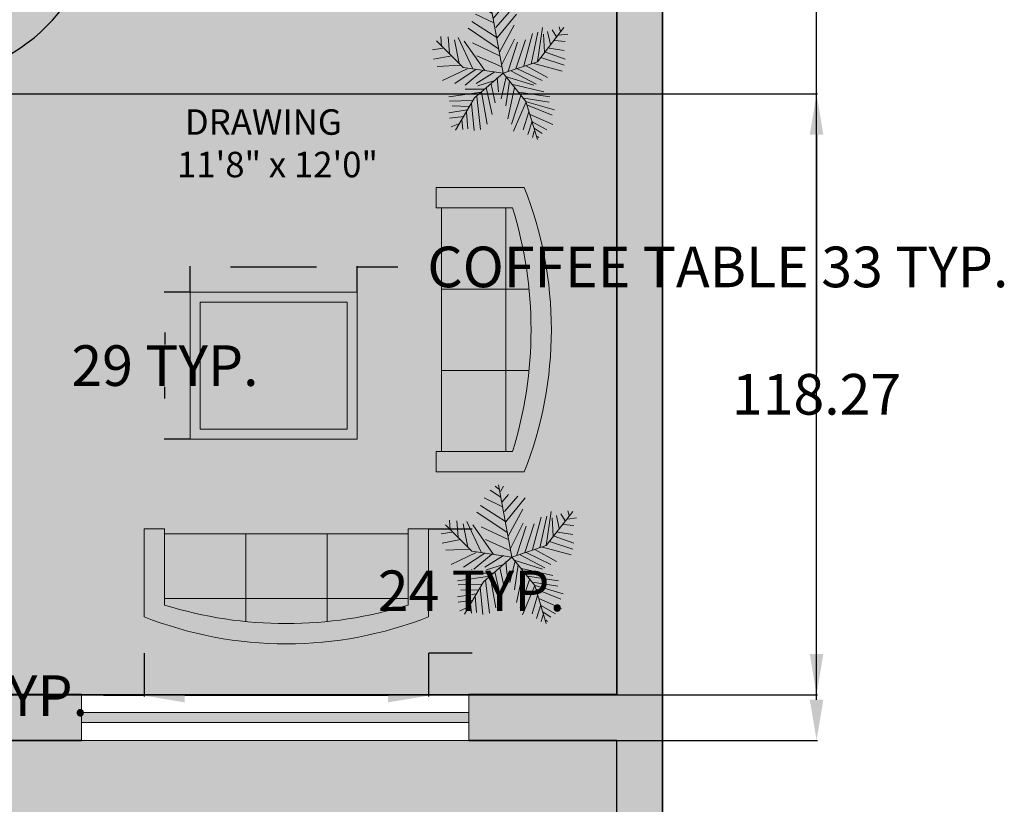
# Model space of a CAD drawing. Units: inches. Extents: x 389 to 971, y 148 to 870.
# Tile 6 of 14: x 722 to 916, y 273 to 428. Entities that reach past the tile are written whole.
import ezdxf

# ---------------------------------------------------------------- set-up
doc = ezdxf.new("R2010")
doc.units = ezdxf.units.IN
doc.header["$MEASUREMENT"] = 0
for name, color, linetype, lineweight in [('A-ANNO-DIMS', 2, 'Continuous', 18), ('A-AREA-IDEN', 7, 'Continuous', 18), ('A-DOOR', 4, 'Continuous', 25), ('A-FLOR-BASE-PATT', 8, 'Continuous', 13), ('A-FURN', 8, 'Continuous', 18), ('A-GLAZ', 4, 'Continuous', 18), ('A-WALL', 7, 'Continuous', 35), ('C-PROP', 7, 'Continuous', 35), ('L-GRND-BASE-PATT', 8, 'Continuous', 13), ('L-PLNT', 3, 'Continuous', 13), ('L-WALL', 7, 'Continuous', 30)]:
    doc.layers.add(name, color=color, linetype=linetype, lineweight=lineweight)
for name, color, linetype, lineweight, true_color in [('A-FURN-SURF-PATT', 9, 'Continuous', 13, 0xd6bdce), ('A-GLAZ-PATT', 251, 'Continuous', 13, 0x6d5f6c), ('A-WALL-PATT', 18, 'Continuous', 13, 0x000000), ('L-GRND-PATT', 39, 'Continuous', 13, 0x603913)]:
    doc.layers.add(name, color=color, linetype=linetype, lineweight=lineweight, true_color=true_color)
doc.styles.get("Standard").update_dxf_attribs({"font": 'arial.ttf'})
doc.dimstyles.get("Standard").update_dxf_attribs({"dimtxt": 8, "dimasz": 8, "dimexe": 0.18, "dimexo": 0.0625, "dimgap": 0.09, "dimtad": 0, "dimtih": 1, "dimtoh": 1, "dimdec": 0, "dimzin": 0, "dimdsep": 46, "dimlunit": 3, "dimtxsty": 'Standard', "dimcen": 0.09, "dimadec": 0, "dimazin": 0, "dimtfac": 1, "dimtdec": 0, "dimtofl": 0, "dimtmove": 0, "dimatfit": 3, "dimfxl": 1, "dimtolj": 1, "dimtzin": 0, "dimarcsym": 0})

# ---------------------------------------------------------------- blocks, each defined once
blk = doc.blocks.new('*U5')
for p, q in [((0, 0), (0, -6)), ((28, 0), (28, -6))]:
    blk.add_line(p, q)
blk.add_lwpolyline([(0, 0), (0, 28), (1.75, 28), (1.75, 0)], close=True)
blk.add_arc((0, 0), 28, 0, 90)
blk = doc.blocks.new('Sofa - Roundback 7 ft.')
for p, q in [((-12.00002, -32.4421), (-12.00003, -6.5971)), ((11.99997, -32.4421), (11.99998, -6.5971)), ((-36.000027, -34), (-36.000027, -11.4696)), ((35.99998, -34), (35.99998, -11.4696)), ((-35.999844, -13.3819), (35.9998, -13.3819)), ((-36.000027, -32.4421), (35.99998, -32.4421))]:
    blk.add_line(p, q)
for points in [[(-36.000027, -34), (-42.000027, -34), (-42.000027, -8)], [(41.99998, -8), (41.99998, -34), (35.99998, -34)]]:
    blk.add_lwpolyline(points)
for centre, radius, start, end in [((0, -114.25), 114.25, 68.43141, 111.5686), ((-0.00001, -127.1968), 121.1968, 72.72033, 107.2797)]:
    blk.add_arc(centre, radius, start, end)
blk = doc.blocks.new('*U19')
for p, q in [((-258.7244, 1362.456), (-332.3336, 1421.4348)), ((0, 0), (-266.7, 1447.8)), ((-231.1146, 1315.2628), (-166.7002, 1421.4348)), ((-185.1152, 1008.5578), (-553.1612, 1185.4942)), ((-221.9198, 1197.3052), (-433.5526, 1338.8594)), ((-194.31, 1102.9442), (-65.4812, 1256.284)), ((-148.3106, 914.1968), (118.5418, 1220.9018)), ((-129.8956, 701.8528), (265.7602, 1185.4942)), ((-129.8956, 713.6638), (-626.7704, 1032.1544)), ((-93.091, 489.5342), (-700.3796, 902.3858)), ((-74.7014, 418.7444), (219.7608, 961.39)), ((412.9786, 147.447), (587.8068, 796.2392)), ((560.197, 182.8292), (698.2206, 819.8358)), ((685.8, 228.6), (1219.2, 914.4)), ((689.0258, 230.0224), (790.2448, 914.1968)), ((891.4384, 831.6214), (946.658, 572.1096)), ((983.4626, 867.0036), (1066.2666, 725.4494)), ((1121.4862, 925.9824), (1149.0706, 831.6214)), ((-800.1, 114.3), (-1333.5, 647.7)), ((-1234.059, 536.7274), (-1252.4486, 737.2604)), ((-1105.2302, 725.4494), (-1077.6458, 395.1732)), ((-976.4268, 666.4706), (-884.4026, 194.6402)), ((-902.8176, 713.6638), (-617.5756, 100.2538)), ((-369.1382, 53.086), (-783.1836, 642.874)), ((-617.5756, 607.4918), (-74.7014, 347.98)), ((-28.6766, 171.0436), (228.9556, 678.2816)), ((100.1268, 41.275), (284.1498, 619.2774)), ((256.5654, 88.4682), (449.7832, 666.4706)), ((808.6344, 784.4282), (827.0494, 418.7444)), ((1029.462, 654.685), (1241.0948, 631.0884)), ((1112.2914, 760.8316), (1296.3144, 784.4282)), ((-1206.4492, 501.3198), (-1418.082, 465.9376)), ((845.439, 418.7444), (1241.0948, 277.1902)), ((919.0482, 501.3198), (1222.6798, 454.152)), ((-1031.621, 347.98), (-1399.667, 277.1902)), ((-525.5514, 347.98), (-28.6766, 123.8504)), ((0, 0), (685.8, 228.6)), ((753.4148, 312.5978), (1222.6798, 159.2326)), ((-847.598, 159.2326), (-1326.0578, 135.636)), ((-718.7946, 88.4682), (-1215.644, -147.447)), ((-543.9664, 76.6572), (-967.2066, -206.4512)), ((0, 0), (-800.1, 114.3)), ((-405.9428, 53.086), (-764.794, -241.8334)), ((0, 0), (-571.5, -495.3)), ((-166.7002, 29.4894), (-543.9664, -206.4512)), ((0, 0), (457.2, -571.5)), ((164.5412, 41.275), (661.416, -218.2368)), ((284.1498, 88.4682), (781.0246, -147.447)), ((458.978, 147.447), (891.4384, -88.4682)), ((615.4166, 194.6402), (1185.8752, 41.275)), ((-166.7002, -147.447), (-507.1618, -253.619)), ((-120.7008, -88.4682), (-93.091, -371.5766)), ((63.3222, -76.6826), (-37.8714, -513.1308)), ((44.9326, -64.897), (615.4166, -241.8334)), ((127.7366, -159.258), (54.1274, -654.685)), ((-442.7474, -383.3876), (-1086.8406, -477.7486)), ((-387.5278, -324.4088), (-764.794, -324.4088)), ((-433.5526, -383.3876), (-323.1134, -1020.3688)), ((-341.5284, -289.0012), (-221.9198, -831.6214)), ((-240.3094, -218.2368), (-157.5054, -595.7062)), ((228.9556, -289.0012), (90.932, -914.1968)), ((192.151, -230.0224), (817.8292, -371.5766)), ((311.7596, -383.3876), (937.4378, -477.7486)), ((-617.5756, -548.5384), (-1077.6458, -560.324)), ((-571.5, -495.3), (-952.5, -1143)), ((-525.5514, -465.963), (-451.9422, -1126.5408)), ((357.759, -430.5554), (164.5412, -1020.3688)), ((458.978, -572.1096), (210.5406, -1161.923)), ((412.9786, -501.3452), (919.0482, -583.9206)), ((457.2, -571.5), (685.8, -1333.5)), ((468.1982, -572.1096), (1029.462, -737.2604)), ((-718.7946, -737.2604), (-1086.8406, -796.2392)), ((-681.9646, -666.496), (-1022.4262, -654.685)), ((-737.1842, -784.4536), (-709.5744, -1114.7298)), ((-635.9652, -607.5172), (-580.771, -1150.1374)), ((514.1976, -772.6426), (403.7838, -1138.3264)), ((486.5878, -642.8994), (983.4626, -843.4324)), ((-783.1836, -867.029), (-1077.6458, -902.4112)), ((-829.2084, -937.7934), (-810.7934, -1126.5408)), ((578.612, -961.39), (495.7826, -1232.7128)), ((541.8074, -831.6214), (992.6574, -1032.1544)), ((578.612, -973.1756), (873.0488, -1138.3264)), ((-875.2078, -1008.5832), (-1040.8412, -1079.3476)), ((624.6114, -1161.923), (587.8068, -1291.6916)), ((624.6114, -1102.9442), (781.0246, -1209.1162)), ((679.8056, -1268.095), (716.6102, -1291.6916))]:
    blk.add_line(p, q)
blk = doc.blocks.new('COFFEE-TABLE-RECT')
for points in [[(0, 28.98), (32.94, 28.98), (32.94, 0), (0, 0)], [(2, 26.98), (30.94, 26.98), (30.94, 2), (2, 2)]]:
    blk.add_lwpolyline(points, close=True)
blk = doc.blocks.new('*D38')
at = {"layer": 'A-ANNO-DIMS', "color": 0, "lineweight": -2, "transparency": 16777216}
for p, q in [((746.14, 302.8), (746.14, 294.28)), ((802.17, 302.8), (802.17, 294.28)), ((746.14, 294.46), (738.14, 294.46)), ((794.17, 294.46), (754.14, 294.46))]:
    blk.add_line(p, q, dxfattribs=at)
at = {"layer": 'A-ANNO-DIMS', "color": 0, "transparency": 16777216}
for points in [[(754.14, 295.79), (754.14, 293.12), (746.14, 294.46)], [(794.17, 295.79), (794.17, 293.12), (802.17, 294.46)]]:
    blk.add_solid(points, dxfattribs=at)
at = {"layer": 'Defpoints', "color": 0, "transparency": 16777216}
for p in [(746.14, 302.86), (802.17, 302.86), (746.14, 294.46)]:
    blk.add_point(p, dxfattribs=at)
at = {"layer": 'A-ANNO-DIMS', "color": 0, "transparency": 16777216, "insert": (701.83, 294.46), "char_height": 8, "attachment_point": 5}
blk.add_mtext('\\A1;SOFA 56 TYP.', dxfattribs=at)
blk = doc.blocks.new('*D39')
at = {"layer": 'A-ANNO-DIMS', "color": 0, "lineweight": -2, "transparency": 16777216}
for p, q in [((802.23, 327.32), (810.76, 327.32)), ((810.58, 319.32), (810.58, 319.2)), ((810.58, 310.86), (810.58, 310.98)), ((802.23, 302.86), (810.76, 302.86))]:
    blk.add_line(p, q, dxfattribs=at)
at = {"layer": 'A-ANNO-DIMS', "color": 0, "transparency": 16777216}
for points in [[(809.24, 319.32), (811.91, 319.32), (810.58, 327.32)], [(809.24, 310.86), (811.91, 310.86), (810.58, 302.86)]]:
    blk.add_solid(points, dxfattribs=at)
at = {"layer": 'Defpoints', "color": 0, "transparency": 16777216}
for p in [(802.17, 327.32), (802.17, 302.86), (810.58, 302.86)]:
    blk.add_point(p, dxfattribs=at)
at = {"layer": 'A-ANNO-DIMS', "color": 0, "transparency": 16777216, "insert": (810.58, 315.09), "char_height": 8, "attachment_point": 5}
blk.add_mtext('\\A1;24 TYP.', dxfattribs=at)
blk = doc.blocks.new('*D42')
at = {"layer": 'A-ANNO-DIMS', "color": 0, "lineweight": -2, "transparency": 16777216}
for p, q in [((755.19, 373.98), (755.19, 379.04)), ((763.19, 378.86), (780.12, 378.86)), ((788.12, 373.98), (788.12, 379.04)), ((788.12, 378.86), (796.12, 378.86))]:
    blk.add_line(p, q, dxfattribs=at)
at = {"layer": 'A-ANNO-DIMS', "color": 0, "transparency": 16777216}
for points in [[(763.19, 380.19), (763.19, 377.52), (755.19, 378.86)], [(780.12, 380.19), (780.12, 377.52), (788.12, 378.86)]]:
    blk.add_solid(points, dxfattribs=at)
at = {"layer": 'Defpoints', "color": 0, "transparency": 16777216}
for p in [(788.12, 378.86), (755.19, 373.92), (788.12, 373.92)]:
    blk.add_point(p, dxfattribs=at)
at = {"layer": 'A-ANNO-DIMS', "color": 0, "transparency": 16777216, "insert": (859.11, 378.86), "char_height": 8, "attachment_point": 5}
blk.add_mtext('\\A1;COFFEE TABLE 33 TYP.', dxfattribs=at)
blk = doc.blocks.new('*D43')
at = {"layer": 'A-ANNO-DIMS', "color": 0, "lineweight": -2, "transparency": 16777216}
for p, q in [((755.12, 373.92), (750.07, 373.92)), ((750.25, 365.92), (750.25, 363.6)), ((750.25, 352.94), (750.25, 355.25)), ((755.12, 344.94), (750.07, 344.94))]:
    blk.add_line(p, q, dxfattribs=at)
at = {"layer": 'A-ANNO-DIMS', "color": 0, "transparency": 16777216}
for points in [[(748.91, 365.92), (751.58, 365.92), (750.25, 373.92)], [(748.91, 352.94), (751.58, 352.94), (750.25, 344.94)]]:
    blk.add_solid(points, dxfattribs=at)
at = {"layer": 'Defpoints', "color": 0, "transparency": 16777216}
for p in [(750.25, 373.92), (755.19, 373.92), (755.19, 344.94)]:
    blk.add_point(p, dxfattribs=at)
at = {"layer": 'A-ANNO-DIMS', "color": 0, "transparency": 16777216, "insert": (750.25, 359.43), "char_height": 8, "attachment_point": 5}
blk.add_mtext('\\A1;29 TYP.', dxfattribs=at)
blk = doc.blocks.new('*D47')
at = {"layer": 'A-ANNO-DIMS', "color": 0, "lineweight": -2, "transparency": 16777216}
for p, q in [((848.28, 834.64), (878.72, 834.64)), ((878.54, 826.64), (878.54, 564.32)), ((878.54, 293.64), (878.54, 555.97)), ((839.28, 285.64), (878.72, 285.64))]:
    blk.add_line(p, q, dxfattribs=at)
at = {"layer": 'A-ANNO-DIMS', "color": 0, "transparency": 16777216}
for points in [[(877.21, 826.64), (879.87, 826.64), (878.54, 834.64)], [(877.21, 293.64), (879.87, 293.64), (878.54, 285.64)]]:
    blk.add_solid(points, dxfattribs=at)
at = {"layer": 'Defpoints', "color": 0, "transparency": 16777216}
for p in [(848.22, 834.64), (878.54, 834.64), (839.22, 285.64)]:
    blk.add_point(p, dxfattribs=at)
at = {"layer": 'A-ANNO-DIMS', "color": 0, "transparency": 16777216, "insert": (878.54, 560.14), "char_height": 8, "attachment_point": 5}
blk.add_mtext('\\A1;549', dxfattribs=at)
blk = doc.blocks.new('*D54')
at = {"layer": 'A-ANNO-DIMS', "color": 0, "lineweight": -2, "transparency": 16777216}
for p, q in [((690.28, 412.92), (878.72, 412.92)), ((878.54, 404.92), (878.54, 357.96)), ((878.54, 302.64), (878.54, 349.61)), ((690.28, 294.64), (878.72, 294.64))]:
    blk.add_line(p, q, dxfattribs=at)
at = {"layer": 'A-ANNO-DIMS', "color": 0, "transparency": 16777216}
for points in [[(877.21, 404.92), (879.87, 404.92), (878.54, 412.92)], [(877.21, 302.64), (879.87, 302.64), (878.54, 294.64)]]:
    blk.add_solid(points, dxfattribs=at)
at = {"layer": 'Defpoints', "color": 0, "transparency": 16777216}
for p in [(690.22, 412.92), (878.54, 412.92), (690.22, 294.64)]:
    blk.add_point(p, dxfattribs=at)
at = {"layer": 'A-ANNO-DIMS', "color": 0, "transparency": 16777216, "insert": (878.54, 353.78), "char_height": 8, "attachment_point": 5}
blk.add_mtext('\\A1;118.27', dxfattribs=at)

msp = doc.modelspace()

# ---------------------------------------------------------------- hatches: boundary and pattern name
at = {"layer": 'A-FLOR-BASE-PATT'}
h = msp.add_hatch(color=256, dxfattribs=at)
h.dxf.hatch_style = 1
h.paths.add_polyline_path([(634.6594, 428.4021), (634.6594, 427.0792), (634.6305, 427.0792, -0.40145271), (604.4225, 398.1652), (604.0817, 398.1199, -0.40145271), (632.0195, 371.3788), (632.0462, 371.3788), (632.0462, 370.1554), (604.387, 370.1554), (604.387, 366.7191), (640.0296, 366.7191), (640.0296, 321.4969, 1), (647.061, 321.4969), (647.061, 412.9189), (690.216, 412.9189), (690.216, 416.0006), (694.716, 416.0006), (702.2145, 416.0006, 0.39601219), (737.1392, 448.8066), (702.2145, 448.8066), (702.2145, 450.9936), (694.716, 450.9936), (690.216, 450.9936), (690.216, 466.6012), (708.7881, 466.6012), (708.7881, 462.1012), (784.6145, 462.1012), (784.6145, 466.6012), (794.216, 466.6012), (794.216, 591.6445), (708.5171, 591.6445), (708.5171, 596.1445), (708.5171, 602.9755, 0.39601219), (678.6314, 634.7912), (678.6314, 602.9755), (676.6391, 602.9755), (676.6391, 596.1445), (676.6391, 591.6445), (661.216, 591.6445), (661.216, 632.6445), (653.109, 632.6445), (653.109, 641.6445), (653.109, 642.1751), (651.6417, 642.1751), (651.6417, 675.6801, 0.40145271), (619.5719, 642.1751), (619.5719, 637.1445), (619.5147, 632.6445), (604.387, 632.6445), (604.387, 545.7317), (595.3894, 545.7317), (595.3894, 544.4199), (565.4338, 544.4199, 0.40145271), (595.3894, 515.7475), (599.887, 515.7475), (604.387, 515.7271), (604.387, 428.4021)])
h.paths.add_polyline_path([(721.8003, 493.9292), (725.0899, 493.9292), (725.0899, 493.075), (751.4065, 493.075), (751.4065, 493.9292), (754.6961, 493.9292), (754.6961, 479.6744, -0.26666697), (721.8003, 479.6744)], flags=16)
h.paths.add_polyline_path([(720.6421, 516.0583), (720.6421, 545.0393), (753.5806, 545.0393), (753.5806, 516.0583)], flags=16)
h.paths.add_polyline_path([(722.6421, 518.0583), (722.6421, 543.0393), (751.5806, 543.0393), (751.5806, 518.0583)], flags=0)
h.paths.add_polyline_path([(763.7396, 488.5801), (763.7822, 488.1156), (764.1436, 488.1761)], flags=16)
h.paths.add_polyline_path([(777.9011, 479.7417), (778.0475, 480.1886), (777.4745, 480.275)], flags=16)
h.paths.add_polyline_path([(762.3329, 503.5919), (762.3329, 507.1718), (763.2624, 507.1718), (763.2624, 550.1306), (762.3329, 550.1306), (762.3329, 553.7105), (777.8458, 553.7105, -0.19047621), (777.8458, 503.5919)], flags=16)
h.paths.add_polyline_path([(721.6097, 567.2898), (721.6097, 581.7362, -0.26666697), (754.9475, 581.7362), (754.9475, 567.2898), (751.6137, 567.2898), (751.6137, 568.1555), (724.9435, 568.1555), (724.9435, 567.2898)], flags=16)
h.paths.add_polyline_path([(774.6347, 521.4914), (774.6347, 535.811), (778.6837, 535.811, -0.04962821), (778.6837, 521.4914)], flags=0)
h.paths.add_polyline_path([(764.6624, 576.8996), (764.7454, 576.4742), (765.0717, 576.4903)], flags=16)
h.paths.add_polyline_path([(777.2772, 570.3652), (777.4444, 570.8756), (776.7899, 570.9743)], flags=16)
h.paths.add_polyline_path([(644.2892, 516.9956), (685.2491, 516.9956), (685.2491, 535.7223), (644.2892, 535.7223)], flags=24)
h = msp.add_hatch(color=256, dxfattribs=at)
h.dxf.hatch_style = 1
h.paths.add_polyline_path([(699.216, 294.6445), (733.8057, 294.6445), (810.0514, 294.6445), (839.216, 294.6445), (839.216, 457.6012), (784.6145, 457.6012), (784.6145, 462.1012), (708.7881, 462.1012), (708.7881, 457.6012), (699.216, 457.6012), (699.216, 450.9936), (702.2145, 450.9936), (737.2076, 450.9936), (737.2076, 448.8066), (737.1392, 448.8066, -0.39601219), (702.2145, 416.0006), (699.216, 416.0006)])
h.paths.add_polyline_path([(755.1859, 373.9163), (788.1244, 373.9163), (788.1244, 344.9352), (755.1859, 344.9352)], flags=16)
h.paths.add_polyline_path([(757.1859, 371.9163), (786.1244, 371.9163), (786.1244, 346.9352), (757.1859, 346.9352)], flags=0)
h.paths.add_polyline_path([(746.1376, 327.3223), (750.14, 327.3223), (750.14, 326.2831), (798.1694, 326.2831), (798.1694, 327.3223), (802.1718, 327.3223), (802.1718, 309.9784, -0.19047621), (746.1376, 309.9784)], flags=16)
h.paths.add_polyline_path([(782.1596, 313.5685), (782.1596, 309.0415, -0.04962821), (766.1498, 309.0415), (766.1498, 313.5685)], flags=0)
h.paths.add_polyline_path([(804.6838, 390.5197), (803.6446, 390.5197), (803.6446, 394.5221), (820.9885, 394.5221, -0.19047621), (820.9885, 338.4879), (803.6446, 338.4879), (803.6446, 342.4903), (804.6838, 342.4903)], flags=16)
h.paths.add_polyline_path([(817.3984, 358.5001), (817.3984, 374.5099), (821.9254, 374.5099, -0.04962821), (821.9254, 358.5001)], flags=0)
h.paths.add_polyline_path([(806.8707, 326.6963), (806.4254, 327.1416), (806.4724, 326.6297)], flags=16)
h.paths.add_polyline_path([(822.0328, 317.4008), (822.1942, 317.8933), (821.5626, 317.9885)], flags=16)
h.paths.add_polyline_path([(808.1446, 418.9737), (808.2247, 418.5632), (808.5395, 418.5787)], flags=16)
h.paths.add_polyline_path([(820.3159, 412.669), (820.4772, 413.1615), (819.8457, 413.2568)], flags=16)
h.paths.add_polyline_path([(750.6082, 393.6667), (791.5681, 393.6667), (791.5681, 412.3933), (750.6082, 412.3933)], flags=24)
at = {"layer": 'A-FURN-SURF-PATT'}
h = msp.add_hatch(color=256, dxfattribs=at)
h.dxf.hatch_style = 1
h.paths.add_polyline_path([(820.9885, 338.4879, 0.19047621), (820.9885, 394.5221), (803.6446, 394.5221), (803.6446, 390.5197), (818.6737, 390.5197, -0.15194781), (818.6737, 342.4903), (803.6446, 342.4903), (803.6446, 338.4879)])
h = msp.add_hatch(color=256, dxfattribs=at)
h.dxf.hatch_style = 1
h.paths.add_polyline_path([(817.3984, 374.5099), (817.3984, 390.5197), (804.6838, 390.5197), (804.6838, 374.5099)])
h = msp.add_hatch(color=256, dxfattribs=at)
h.dxf.hatch_style = 1
h.paths.add_polyline_path([(818.6737, 390.5197), (817.3984, 390.5197), (817.3984, 374.5099), (821.9254, 374.5099, 0.05064665)])
h = msp.add_hatch(color=256, dxfattribs=at)
h.dxf.hatch_style = 1
h.paths.add_polyline_path([(817.3984, 374.5099), (804.6838, 374.5099), (804.6838, 358.5001), (817.3984, 358.5001)])
h = msp.add_hatch(color=256, dxfattribs=at)
h.dxf.hatch_style = 1
h.paths.add_polyline_path([(821.9254, 374.5099), (817.3984, 374.5099), (817.3984, 358.5001), (821.9254, 358.5001, 0.04962821)])
h = msp.add_hatch(color=256, dxfattribs=at)
h.dxf.hatch_style = 1
h.paths.add_polyline_path([(788.1244, 373.9163), (755.1859, 373.9163), (755.1859, 344.9352), (788.1244, 344.9352)])
h.paths.add_polyline_path([(786.1244, 346.9352), (757.1859, 346.9352), (757.1859, 371.9163), (786.1244, 371.9163)], flags=16)
h = msp.add_hatch(color=256, dxfattribs=at)
h.dxf.hatch_style = 1
h.paths.add_polyline_path([(786.1244, 346.9352), (786.1244, 371.9163), (757.1859, 371.9163), (757.1859, 346.9352)])
h = msp.add_hatch(color=256, dxfattribs=at)
h.dxf.hatch_style = 1
h.paths.add_polyline_path([(804.6838, 342.4903), (817.3984, 342.4903), (817.3984, 358.5001), (804.6838, 358.5001)])
h = msp.add_hatch(color=256, dxfattribs=at)
h.dxf.hatch_style = 1
h.paths.add_polyline_path([(821.9254, 358.5001), (817.3984, 358.5001), (817.3984, 342.4903), (818.6737, 342.4903, 0.05064665)])
h = msp.add_hatch(color=256, dxfattribs=at)
h.dxf.hatch_style = 1
h.paths.add_polyline_path([(802.1718, 309.9784), (802.1718, 327.3223), (798.1694, 327.3223), (798.1694, 312.2932, -0.15194781), (750.14, 312.2932), (750.14, 327.3223), (746.1376, 327.3223), (746.1376, 309.9784, 0.19047621)])
h = msp.add_hatch(color=256, dxfattribs=at)
h.dxf.hatch_style = 1
h.paths.add_polyline_path([(750.14, 326.2831), (750.14, 313.5685), (766.1498, 313.5685), (766.1498, 326.2831)])
h = msp.add_hatch(color=256, dxfattribs=at)
h.dxf.hatch_style = 1
h.paths.add_polyline_path([(766.1498, 313.5685), (782.1596, 313.5685), (782.1596, 326.2831), (766.1498, 326.2831)])
h = msp.add_hatch(color=256, dxfattribs=at)
h.dxf.hatch_style = 1
h.paths.add_polyline_path([(798.1694, 313.5685), (798.1694, 326.2831), (782.1596, 326.2831), (782.1596, 313.5685)])
h = msp.add_hatch(color=256, dxfattribs=at)
h.dxf.hatch_style = 1
h.paths.add_polyline_path([(750.14, 313.5685), (750.14, 312.2932, 0.05064665), (766.1498, 309.0415), (766.1498, 313.5685)])
h = msp.add_hatch(color=256, dxfattribs=at)
h.dxf.hatch_style = 1
h.paths.add_polyline_path([(766.1498, 313.5685), (766.1498, 309.0415, 0.04962821), (782.1596, 309.0415), (782.1596, 313.5685)])
h = msp.add_hatch(color=256, dxfattribs=at)
h.dxf.hatch_style = 1
h.paths.add_polyline_path([(798.1694, 312.2932), (798.1694, 313.5685), (782.1596, 313.5685), (782.1596, 309.0415, 0.05064665)])
at = {"layer": 'A-GLAZ-PATT'}
h = msp.add_hatch(color=256, dxfattribs=at)
h.dxf.hatch_style = 1
h.paths.add_polyline_path([(733.8057, 291.1445), (733.8057, 289.1445), (810.0514, 289.1445), (810.0514, 291.1445)])
h = msp.add_hatch(color=256, dxfattribs=at)
h.dxf.hatch_style = 1
h.paths.add_polyline_path([(733.8057, 291.1445), (733.8057, 289.1445), (810.0514, 289.1445), (810.0514, 291.1445)])
h = msp.add_hatch(color=256, dxfattribs=at)
h.dxf.hatch_style = 1
h.paths.add_polyline_path([(810.0514, 289.1445), (810.0514, 291.1445), (733.8057, 291.1445), (733.8057, 289.1445)])
h = msp.add_hatch(color=256, dxfattribs=at)
h.dxf.hatch_style = 1
h.paths.add_polyline_path([(733.8057, 291.1445), (733.8057, 289.1445), (810.0514, 289.1445), (810.0514, 291.1445)])
h = msp.add_hatch(color=256, dxfattribs=at)
h.dxf.hatch_style = 1
h.paths.add_polyline_path([(733.8057, 291.1445), (733.8057, 289.1445), (810.0514, 289.1445), (810.0514, 291.1445)])
at = {"layer": 'A-WALL-PATT'}
h = msp.add_hatch(color=256, dxfattribs=at)
h.dxf.hatch_style = 1
h.paths.add_polyline_path([(432.216, 434.6445), (436.3673, 434.6445), (436.3673, 443.6445), (432.216, 443.6445), (432.216, 830.6445), (746.216, 830.6445), (746.216, 823.8175), (755.216, 823.8175), (755.216, 825.6445), (839.216, 825.6445), (839.216, 803.5176), (839.216, 741.6445), (755.216, 741.6445), (755.216, 748.4596), (755.1859, 748.4596), (750.716, 748.4596), (746.216, 748.4596), (746.216, 732.6445), (839.216, 732.6445), (839.216, 600.6445), (708.5171, 600.6445), (708.5171, 596.1445), (708.5171, 591.6445), (794.216, 591.6445), (794.216, 587.4291), (803.216, 587.4291), (803.216, 591.6445), (839.216, 591.6445), (839.216, 466.6012), (803.216, 466.6012), (803.216, 471.0309), (794.216, 471.0309), (794.216, 466.6012), (784.6145, 466.6012), (784.6145, 457.6012), (839.216, 457.6012), (839.216, 447.6445), (839.216, 294.6445), (810.0514, 294.6445), (810.0514, 285.6445), (839.216, 285.6445), (839.216, 238.6445), (590.216, 238.6445), (590.216, 234.6445), (848.216, 234.6445), (848.216, 834.6445), (428.216, 834.6445), (428.216, 234.6445), (437.216, 234.6445), (437.216, 243.6445), (432.216, 243.6445)])
h = msp.add_hatch(color=256, dxfattribs=at)
h.dxf.hatch_style = 1
h.paths.add_polyline_path([(690.216, 294.6445), (684.2434, 294.6445), (684.2434, 285.6445), (733.8057, 285.6445), (733.8057, 294.6445), (699.216, 294.6445), (699.216, 416.0006), (694.716, 416.0006), (690.216, 416.0006)])
h = msp.add_hatch(color=256, dxfattribs=at)
h.dxf.hatch_style = 1
h.paths.add_polyline_path([(690.216, 294.6445), (684.2434, 294.6445), (684.2434, 285.6445), (733.8057, 285.6445), (733.8057, 294.6445), (699.216, 294.6445), (699.216, 400.9189), (690.216, 400.9189)])
at = {"layer": 'L-GRND-BASE-PATT'}
h = msp.add_hatch(color=256, dxfattribs=at)
h.dxf.hatch_style = 1
edge = h.paths.add_edge_path(flags=16)
edge.add_ellipse((8782.0026, 354.2473), major_axis=(-8296.9493, 0), ratio=0.84230387, start_angle=-0.09022909, end_angle=0.38386678, ccw=False)
edge.add_ellipse((485.0533, 368.2895), major_axis=(-1.1591, 0), ratio=0.84230387, start_angle=0, end_angle=90, ccw=False)
edge.add_line((483.8943, 368.2895), (483.8943, 387.6039))
edge.add_ellipse((485.0533, 387.2466), major_axis=(1.1591, 0), ratio=0.84230387, start_angle=90, end_angle=180, ccw=False)
edge.add_line((485.0533, 388.2229), (485.5047, 388.2229))
edge.add_ellipse((898.8202, 372.4897), major_axis=(413.7374, 0), ratio=0.84230387, start_angle=176.349572, end_angle=177.82005, ccw=False)
edge.add_ellipse((535.9119, 196.3855), major_axis=(-245.3972, 0), ratio=0.84230387, start_angle=-77.874034, end_angle=-76.219471, ccw=False)
edge.add_ellipse((535.9119, 201.7547), major_axis=(239.1274, 0), ratio=0.84230387, start_angle=100.209539, end_angle=102.444627, ccw=False)
edge.add_ellipse((473.3139, 564.9222), major_axis=(196.5637, 0), ratio=0.84230387, start_angle=-80.743434, end_angle=-77.445067)
edge.add_line((509.5535, 402.1941), (514.3535, 404.8483))
edge.add_line((514.3535, 404.8483), (514.3535, 404.7972))
edge.add_ellipse((514.3535, 404.2644), major_axis=(0.5795, 0), ratio=0.84230387, start_angle=52.06687, end_angle=90, ccw=False)
edge.add_line((514.6716, 404.6725), (519.1535, 402.1941))
edge.add_ellipse((555.3932, 564.9222), major_axis=(-196.5637, 0), ratio=0.84230387, start_angle=77.445067, end_angle=80.743434)
edge.add_ellipse((492.7951, 201.7547), major_axis=(239.1274, 0), ratio=0.84230387, start_angle=77.555373, end_angle=79.790461, ccw=False)
edge.add_ellipse((492.7951, 196.3855), major_axis=(245.3972, 0), ratio=0.84230387, start_angle=76.219471, end_angle=77.874034, ccw=False)
edge.add_ellipse((129.8868, 372.4897), major_axis=(-413.7374, 0), ratio=0.84230387, start_angle=182.17995, end_angle=183.650428, ccw=False)
edge.add_line((543.2023, 388.2229), (544.0779, 388.2229))
edge.add_ellipse((543.6537, 387.2466), major_axis=(-1.1591, 0), ratio=0.84230387, start_angle=180, end_angle=270, ccw=False)
edge.add_line((544.8128, 387.2466), (544.8128, 367.9322))
edge.add_ellipse((543.6537, 368.2895), major_axis=(1.1591, 0), ratio=0.84230387, start_angle=270, end_angle=360, ccw=False)
edge.add_ellipse((-7753.2956, 354.2473), major_axis=(-8296.9493, 0), ratio=0.84230387, start_angle=179.61613322, end_angle=180.09022909, ccw=False)
edge.add_line((543.3912, 298.6608), (544.0779, 298.6608))
edge.add_ellipse((543.6537, 297.6845), major_axis=(1.1591, 0), ratio=0.84230387, start_angle=0, end_angle=90, ccw=False)
edge.add_line((544.8128, 297.6845), (544.8128, 278.3701))
edge.add_ellipse((543.6537, 278.7275), major_axis=(-1.1591, 0), ratio=0.84230387, start_angle=90, end_angle=180, ccw=False)
edge.add_line((543.6537, 277.7512), (543.1566, 277.7512))
edge.add_ellipse((-7753.2956, 354.2473), major_axis=(-8296.9493, 0), ratio=0.84230387, start_angle=179.3813568, end_angle=179.47172853, ccw=False)
edge.add_ellipse((542.4236, 263.2763), major_axis=(-1.7386, 0), ratio=0.84230387, start_angle=179.371763, end_angle=248.464757, ccw=False)
edge.add_ellipse((-7753.8751, 354.2473), major_axis=(-8298.7403, 0), ratio=0.842303866, start_angle=179.35344592, end_angle=179.3717628, ccw=False)
edge.add_ellipse((540.0116, 260.6509), major_axis=(-4.1092, 0), ratio=0.84230387, start_angle=90, end_angle=179.353446, ccw=False)
edge.add_line((540.0116, 257.1897), (488.6954, 257.1897))
edge.add_ellipse((488.6954, 260.6509), major_axis=(4.1092, 0), ratio=0.84230387, start_angle=180.646554, end_angle=270, ccw=False)
edge.add_ellipse((8782.5821, 354.2473), major_axis=(-8298.7403, 0), ratio=0.842303872, start_angle=0.62823723, end_angle=0.64655411, ccw=False)
edge.add_ellipse((486.2834, 263.2763), major_axis=(-1.7386, 0), ratio=0.84230387, start_angle=-68.464756, end_angle=0.628237, ccw=False)
edge.add_ellipse((8782.0026, 354.2473), major_axis=(-8296.9493, 0), ratio=0.84230387, start_angle=0.52827147, end_angle=0.6465541, ccw=False)
edge.add_line((485.5504, 277.7512), (484.6291, 277.7512))
edge.add_ellipse((485.0533, 278.7275), major_axis=(-1.1591, 0), ratio=0.84230387, start_angle=0, end_angle=90, ccw=False)
edge.add_line((483.8943, 278.7275), (483.8943, 298.0418))
edge.add_ellipse((485.0533, 297.6845), major_axis=(1.1591, 0), ratio=0.84230387, start_angle=90, end_angle=180, ccw=False)
edge = h.paths.add_edge_path(flags=0)
edge.add_ellipse((8782.0026, 354.2473), major_axis=(-8295.7902, 0), ratio=0.84230387, start_angle=0.05559431, end_angle=0.37776419, ccw=False)
edge.add_line((486.2179, 346.1978), (489.3905, 335.8384))
edge.add_ellipse((3386.0114, 329.7263), major_axis=(-2896.63, 0), ratio=0.84230387, start_angle=-0.1208974, end_angle=0.3640763)
edge.add_line((489.4638, 311.3204), (486.4666, 299.5521))
edge = h.paths.add_edge_path(flags=0)
edge.add_ellipse((514.3535, 391.3731), major_axis=(-115.1513, 0), ratio=0.84230387, start_angle=76.401865, end_angle=103.598135)
edge.add_line((537.3428, 296.3333), (537.3428, 281.5897))
edge.add_ellipse((514.3535, 376.6295), major_axis=(-115.1513, 0), ratio=0.84230387, start_angle=76.401865, end_angle=103.598135, ccw=False)
edge.add_line((491.3643, 281.5897), (491.3643, 296.3333))
edge = h.paths.add_edge_path(flags=0)
edge.add_line((491.3643, 337.0752), (489.653, 349.9016))
edge.add_ellipse((510.1338, 298.7862), major_axis=(64.0481, 0), ratio=0.84230387, start_angle=94.277421, end_angle=111.834954, ccw=False)
edge.add_line((506.1068, 352.6274), (522.6002, 352.6274))
edge.add_ellipse((518.5732, 298.7862), major_axis=(64.0481, 0), ratio=0.84230387, start_angle=68.165046, end_angle=85.722579, ccw=False)
edge.add_line((539.0541, 349.9016), (537.3428, 337.0752))
edge.add_ellipse((516.5462, 287.5825), major_axis=(62.3305, 0), ratio=0.84230387, start_angle=67.208085, end_angle=85.12993)
edge.add_line((521.008, 339.949), (507.699, 339.949))
edge.add_ellipse((512.1609, 287.5825), major_axis=(62.3305, 0), ratio=0.84230387, start_angle=94.87007, end_angle=112.791915)
edge = h.paths.add_edge_path(flags=0)
edge.add_ellipse((493.6824, 273.9439), major_axis=(-2.3182, 0), ratio=0.84230387, start_angle=-90, end_angle=0, ccw=False)
edge.add_line((493.6824, 275.8965), (535.3743, 275.8965))
edge.add_ellipse((535.0246, 273.9439), major_axis=(2.3182, 0), ratio=0.84230387, start_angle=0, end_angle=90, ccw=False)
edge.add_line((537.3428, 273.9439), (537.3428, 258.6983))
edge.add_line((537.3428, 258.6983), (540.5912, 258.6983))
edge.add_ellipse((540.5912, 260.6509), major_axis=(-2.3182, 0), ratio=0.84230387, start_angle=90, end_angle=179.353446)
edge.add_line((540.5912, 258.6983), (487.7691, 258.6983))
edge.add_ellipse((488.1158, 260.6509), major_axis=(2.3182, 0), ratio=0.84230387, start_angle=180.646554, end_angle=270)
edge.add_line((488.1158, 258.6983), (491.3643, 258.6983))
edge.add_line((491.3643, 258.6983), (491.3643, 274.2384))
h.paths.add_polyline_path([(746.1376, 327.3223), (750.14, 327.3223), (750.14, 326.2831), (798.1694, 326.2831), (798.1694, 327.3223), (802.1718, 327.3223), (802.1718, 309.9784, -0.19047621), (746.1376, 309.9784)], flags=16)
h.paths.add_polyline_path([(782.1596, 313.5685), (782.1596, 309.0415, -0.04962821), (766.1498, 309.0415), (766.1498, 313.5685)], flags=0)
h.paths.add_polyline_path([(755.1859, 344.9352), (755.1859, 373.9163), (788.1244, 373.9163), (788.1244, 344.9352)], flags=16)
h.paths.add_polyline_path([(757.1859, 346.9352), (757.1859, 371.9163), (786.1244, 371.9163), (786.1244, 346.9352)], flags=0)
h.paths.add_polyline_path([(803.6446, 338.4879), (803.6446, 342.4903), (804.6838, 342.4903), (804.6838, 390.5197), (803.6446, 390.5197), (803.6446, 394.5221), (820.9885, 394.5221, -0.19047621), (820.9885, 338.4879)], flags=16)
h.paths.add_polyline_path([(806.8707, 326.6963), (806.4254, 327.1416), (806.4724, 326.6297)], flags=16)
h.paths.add_polyline_path([(822.0328, 317.4008), (822.1942, 317.8933), (821.5626, 317.9885)], flags=16)
h.paths.add_polyline_path([(817.3984, 358.5001), (817.3984, 374.5099), (821.9254, 374.5099, -0.04962821), (821.9254, 358.5001)], flags=0)
h.paths.add_polyline_path([(808.1446, 418.9737), (808.2247, 418.5632), (808.5395, 418.5787)], flags=16)
h.paths.add_polyline_path([(820.3159, 412.669), (820.4772, 413.1615), (819.8457, 413.2568)], flags=16)
h.paths.add_polyline_path([(466.3155, 235.5246), (517.3807, 235.5246), (517.3807, 244.4269), (466.3155, 244.4269)], flags=24)
h.paths.add_polyline_path([(739.8737, 256.2), (815.404, 256.2), (815.404, 265.3454), (739.8737, 265.3454)], flags=24)
h.paths.add_polyline_path([(750.6082, 393.6667), (791.5681, 393.6667), (791.5681, 412.3933), (750.6082, 412.3933)], flags=24)
h.paths.add_polyline_path([(438.9631, 410.0619), (484.6204, 410.0619), (484.6204, 429.1217), (438.9631, 429.1217)], flags=24)
edge = h.paths.add_edge_path()
edge.add_line((839.216, 285.6445), (611.8787, 285.6445))
edge.add_line((611.8787, 285.6445), (604.387, 285.6445))
edge.add_line((604.387, 285.6445), (595.387, 285.6445))
edge.add_line((595.387, 285.6445), (595.387, 370.1554))
edge.add_line((595.387, 370.1554), (604.0817, 370.1554))
edge.add_line((604.0817, 370.1554), (604.0817, 371.3788))
edge.add_line((604.0817, 371.3788), (632.0195, 371.3788))
edge.add_arc((604.0817, 370.1554), 27.9645, 2.507491, 90)
edge.add_line((604.0817, 398.1199), (599.887, 398.1652))
edge.add_line((599.887, 398.1652), (604.4225, 398.1652))
edge.add_arc((604.4225, 428.4021), 30.2369, 270, 357.492509)
edge.add_line((634.6305, 427.0792), (604.4225, 427.0792))
edge.add_line((604.4225, 427.0792), (604.4225, 428.4021))
edge.add_line((604.4225, 428.4021), (599.887, 428.4021))
edge.add_line((599.887, 428.4021), (595.387, 428.4021))
edge.add_line((595.387, 428.4021), (595.387, 434.6445))
edge.add_line((595.387, 434.6445), (585.0791, 434.6445))
edge.add_line((585.0791, 434.6445), (540.3922, 434.6445))
edge.add_line((540.3922, 434.6445), (526.7125, 434.6445))
edge.add_line((526.7125, 434.6445), (488.4095, 434.6445))
edge.add_line((488.4095, 434.6445), (432.216, 434.6445))
edge.add_line((432.216, 434.6445), (432.216, 243.6445))
edge.add_line((432.216, 243.6445), (437.216, 243.6445))
edge.add_line((437.216, 243.6445), (437.216, 234.6445))
edge.add_line((437.216, 234.6445), (581.216, 234.6445))
edge.add_line((581.216, 234.6445), (581.216, 238.6445))
edge.add_line((581.216, 238.6445), (581.216, 243.6445))
edge.add_line((581.216, 243.6445), (590.216, 243.6445))
edge.add_line((590.216, 243.6445), (590.216, 238.6445))
edge.add_line((590.216, 238.6445), (839.216, 238.6445))
edge.add_line((839.216, 238.6445), (839.216, 285.6445))
at = {"layer": 'L-GRND-PATT'}
h = msp.add_hatch(dxfattribs=at)
h.set_pattern_fill('EARTH', color=256, angle=45)
h.set_pattern_definition([(45, (0, 0), (0, 8.980256), [6.35, -6.35]), (45, (-1.684, 1.684), (0, 8.980256), [6.35, -6.35]), (45, (-3.3676, 3.3676), (0, 8.980256), [6.35, -6.35]), (135, (-3.3676, 4.49), (-8.980256, 0), [6.35, -6.35]), (135, (-1.684, 6.174), (-8.980256, 0), [6.35, -6.35]), (135, (0, 7.858), (-8.980256, 0), [6.35, -6.35])])
h.paths.add_polyline_path([(432.216, 243.6445), (437.216, 243.6445), (437.216, 234.6445), (581.216, 234.6445), (581.216, 238.6445), (581.216, 243.6445), (590.216, 243.6445), (590.216, 238.6445), (839.216, 238.6445), (839.216, 285.6445), (810.0514, 285.6445), (733.8057, 285.6445), (684.2434, 285.6445), (611.8787, 285.6445), (604.387, 285.6445), (595.387, 285.6445), (595.387, 370.1554), (604.0817, 370.1554), (604.0817, 371.3788), (632.0195, 371.3788, 0.40145271), (604.0817, 398.1199), (599.887, 398.1652), (604.4225, 398.1652, 0.40145271), (634.6305, 427.0792), (604.4225, 427.0792), (604.4225, 428.4021), (599.887, 428.4021), (595.387, 428.4021), (595.387, 434.6445), (585.0791, 434.6445), (540.3922, 434.6445), (526.7125, 434.6445), (488.4095, 434.6445), (432.216, 434.6445)])
edge = h.paths.add_edge_path(flags=16)
edge.add_line((483.8943, 278.7275), (483.8943, 298.2564))
edge.add_ellipse((485.0533, 297.6845), major_axis=(1.1591, 0), ratio=0.84230387, start_angle=90, end_angle=180, ccw=False)
edge.add_ellipse((8782.0026, 354.2473), major_axis=(-8296.9493, 0), ratio=0.84230387, start_angle=-0.09022909, end_angle=0.38386678, ccw=False)
edge.add_ellipse((485.0533, 368.2895), major_axis=(-1.1591, 0), ratio=0.84230387, start_angle=0, end_angle=90, ccw=False)
edge.add_line((483.8943, 368.2895), (483.8943, 387.8185))
edge.add_ellipse((485.0533, 387.2466), major_axis=(1.1591, 0), ratio=0.84230387, start_angle=90, end_angle=180, ccw=False)
edge.add_ellipse((898.8202, 372.4897), major_axis=(413.7374, 0), ratio=0.84230387, start_angle=176.349572, end_angle=177.82005, ccw=False)
edge.add_ellipse((535.9119, 196.3855), major_axis=(-245.3972, 0), ratio=0.84230387, start_angle=-77.874034, end_angle=-76.219471, ccw=False)
edge.add_ellipse((535.9119, 201.7547), major_axis=(239.1274, 0), ratio=0.84230387, start_angle=100.209539, end_angle=102.444627, ccw=False)
edge.add_ellipse((473.3139, 564.9222), major_axis=(196.5637, 0), ratio=0.84230387, start_angle=-80.743434, end_angle=-77.445067)
edge.add_line((509.5535, 402.1941), (514.3535, 404.8483))
edge.add_line((514.3535, 404.8483), (519.1535, 402.1941))
edge.add_ellipse((555.3932, 564.9222), major_axis=(-196.5637, 0), ratio=0.84230387, start_angle=77.445067, end_angle=80.743434)
edge.add_ellipse((492.7951, 201.7547), major_axis=(239.1274, 0), ratio=0.84230387, start_angle=77.555373, end_angle=79.790461, ccw=False)
edge.add_ellipse((492.7951, 196.3855), major_axis=(245.3972, 0), ratio=0.84230387, start_angle=76.219471, end_angle=77.874034, ccw=False)
edge.add_ellipse((129.8868, 372.4897), major_axis=(-413.7374, 0), ratio=0.84230387, start_angle=182.17995, end_angle=183.650428, ccw=False)
edge.add_line((543.2023, 388.2229), (544.3327, 388.2229))
edge.add_ellipse((543.6537, 387.2466), major_axis=(-1.1591, 0), ratio=0.84230387, start_angle=180, end_angle=270, ccw=False)
edge.add_line((544.8128, 387.2466), (544.8128, 367.7176))
edge.add_ellipse((543.6537, 368.2895), major_axis=(1.1591, 0), ratio=0.84230387, start_angle=270, end_angle=360, ccw=False)
edge.add_ellipse((-7753.2956, 354.2473), major_axis=(-8296.9493, 0), ratio=0.84230387, start_angle=179.61613322, end_angle=180.09022909, ccw=False)
edge.add_ellipse((543.6537, 297.6845), major_axis=(1.1591, 0), ratio=0.84230387, start_angle=0, end_angle=90, ccw=False)
edge.add_line((544.8128, 297.6845), (544.8128, 278.1556))
edge.add_ellipse((543.6537, 278.7275), major_axis=(-1.1591, 0), ratio=0.84230387, start_angle=90, end_angle=180, ccw=False)
edge.add_ellipse((-7753.2956, 354.2473), major_axis=(-8296.9493, 0), ratio=0.84230387, start_angle=179.3813568, end_angle=179.47172853, ccw=False)
edge.add_ellipse((542.4236, 263.2763), major_axis=(-1.7386, 0), ratio=0.84230387, start_angle=179.371763, end_angle=248.464757, ccw=False)
edge.add_ellipse((-7753.8751, 354.2473), major_axis=(-8298.7403, 0), ratio=0.842303866, start_angle=179.35344592, end_angle=179.3717628, ccw=False)
edge.add_ellipse((540.0116, 260.6509), major_axis=(-4.1092, 0), ratio=0.84230387, start_angle=90, end_angle=179.353446, ccw=False)
edge.add_line((540.0116, 257.1897), (488.0808, 257.1897))
edge.add_ellipse((488.6954, 260.6509), major_axis=(4.1092, 0), ratio=0.84230387, start_angle=180.646554, end_angle=270, ccw=False)
edge.add_ellipse((8782.5821, 354.2473), major_axis=(-8298.7403, 0), ratio=0.842303872, start_angle=0.62823723, end_angle=0.64655411, ccw=False)
edge.add_ellipse((486.2834, 263.2763), major_axis=(-1.7386, 0), ratio=0.84230387, start_angle=-68.464756, end_angle=0.628237, ccw=False)
edge.add_ellipse((8782.0026, 354.2473), major_axis=(-8296.9493, 0), ratio=0.84230387, start_angle=0.52827147, end_angle=0.6465541, ccw=False)
edge.add_line((485.5504, 277.7512), (484.3744, 277.7512))
edge.add_ellipse((485.0533, 278.7275), major_axis=(-1.1591, 0), ratio=0.84230387, start_angle=0, end_angle=90, ccw=False)
edge = h.paths.add_edge_path(flags=0)
edge.add_ellipse((488.1158, 260.6509), major_axis=(2.3182, 0), ratio=0.84230387, start_angle=180.646554, end_angle=270)
edge.add_line((488.1158, 258.6983), (491.3643, 258.6983))
edge.add_line((491.3643, 258.6983), (491.3643, 274.4686))
edge.add_ellipse((493.6824, 273.9439), major_axis=(-2.3182, 0), ratio=0.84230387, start_angle=-90, end_angle=0, ccw=False)
edge.add_line((493.6824, 275.8965), (535.6476, 275.8965))
edge.add_ellipse((535.0246, 273.9439), major_axis=(2.3182, 0), ratio=0.84230387, start_angle=0, end_angle=90, ccw=False)
edge.add_line((537.3428, 273.9439), (537.3428, 258.6983))
edge.add_line((537.3428, 258.6983), (541.2086, 258.6983))
edge.add_ellipse((540.5912, 260.6509), major_axis=(-2.3182, 0), ratio=0.84230387, start_angle=90, end_angle=179.353446, ccw=False)
edge.add_line((540.5912, 258.6983), (487.4984, 258.6983))
edge = h.paths.add_edge_path(flags=0)
edge.add_line((491.3643, 281.5897), (491.3643, 296.3333))
edge.add_ellipse((514.3535, 391.3731), major_axis=(-115.1513, 0), ratio=0.84230387, start_angle=76.401865, end_angle=103.598135)
edge.add_line((537.3428, 296.3333), (537.3428, 281.5897))
edge.add_ellipse((514.3535, 376.6295), major_axis=(-115.1513, 0), ratio=0.84230387, start_angle=76.401865, end_angle=103.598135, ccw=False)
edge = h.paths.add_edge_path(flags=0)
edge.add_ellipse((8782.0026, 354.2473), major_axis=(-8295.7902, 0), ratio=0.84230387, start_angle=0.05559431, end_angle=0.37776419, ccw=False)
edge.add_line((486.2179, 346.1978), (489.3905, 335.8384))
edge.add_ellipse((3386.0114, 329.7263), major_axis=(-2896.63, 0), ratio=0.84230387, start_angle=-0.1208974, end_angle=0.3640763)
edge.add_line((489.4638, 311.3204), (486.4666, 299.5521))
edge = h.paths.add_edge_path(flags=0)
edge.add_line((491.3643, 337.0752), (489.653, 349.9016))
edge.add_ellipse((510.1338, 298.7862), major_axis=(64.0481, 0), ratio=0.84230387, start_angle=94.277421, end_angle=111.834954, ccw=False)
edge.add_line((506.1068, 352.6274), (522.6002, 352.6274))
edge.add_ellipse((518.5732, 298.7862), major_axis=(64.0481, 0), ratio=0.84230387, start_angle=68.165046, end_angle=85.722579, ccw=False)
edge.add_line((539.0541, 349.9016), (537.3428, 337.0752))
edge.add_ellipse((516.5462, 287.5825), major_axis=(62.3305, 0), ratio=0.84230387, start_angle=67.208085, end_angle=85.12993)
edge.add_line((521.008, 339.949), (507.699, 339.949))
edge.add_ellipse((512.1609, 287.5825), major_axis=(62.3305, 0), ratio=0.84230387, start_angle=94.87007, end_angle=112.791915)
h.paths.add_polyline_path([(466.3155, 235.5246), (517.3807, 235.5246), (517.3807, 244.4269), (466.3155, 244.4269)], flags=24)
h.paths.add_polyline_path([(739.8737, 256.2), (815.404, 256.2), (815.404, 265.3454), (739.8737, 265.3454)], flags=24)
h.paths.add_polyline_path([(438.9631, 410.0619), (484.6204, 410.0619), (484.6204, 429.1217), (438.9631, 429.1217)], flags=24)

# ---------------------------------------------------------------- linework, layer by layer
at = {"layer": 'A-GLAZ'}
for p, q in [((733.8057, 294.6445), (733.8057, 285.6445)), ((733.8057, 294.6445), (810.0514, 294.6445)), ((810.0514, 294.6445), (810.0514, 285.6445)), ((810.0514, 294.6445), (810.0514, 285.6445)), ((733.8057, 291.1445), (810.0514, 291.1445)), ((733.8057, 289.1445), (810.0514, 289.1445)), ((733.8057, 285.6445), (810.0514, 285.6445))]:
    msp.add_line(p, q, dxfattribs=at)
at = {"layer": 'A-WALL'}
for p, q in [((839.216, 294.6445), (839.216, 457.6012)), ((733.8057, 294.6445), (699.216, 294.6445)), ((839.216, 294.6445), (810.0514, 294.6445)), ((733.8057, 285.6445), (684.2434, 285.6445)), ((839.216, 285.6445), (810.0514, 285.6445))]:
    msp.add_line(p, q, dxfattribs=at)
at = {"layer": 'C-PROP'}
msp.add_line((848.216, 234.6445), (848.216, 834.6445), dxfattribs=at)
at = {"layer": 'L-WALL'}
msp.add_line((839.216, 238.6445), (839.216, 285.6445), dxfattribs=at)

# ---------------------------------------------------------------- block references
at = {"layer": 'A-DOOR', "xscale": 1.249752530320971, "yscale": 1.249752530320971, "zscale": 1.249752530320971, "rotation": 270}
msp.add_blockref('*U5', (702.2145, 450.9936), dxfattribs=at)
at = {"layer": 'A-FURN'}
for p, xscale, yscale, zscale, rotation in [((826.3251, 366.505), 0.6670743320704638, 0.6670743320704638, 0.6670743320704638, 270), ((774.1547, 304.6418), 0.6670743320704624, 0.6670743320704624, 0.6670743320704624, 180)]:
    msp.add_blockref('Sofa - Roundback 7 ft.', p, dxfattribs=dict(at, xscale=xscale, yscale=yscale, zscale=zscale, rotation=rotation))
msp.add_blockref('COFFEE-TABLE-RECT', (755.1859, 344.9352), dxfattribs=at)
at = {"layer": 'L-PLNT', "xscale": 0.0098214307456944, "yscale": 0.0098214307456944, "zscale": 0.0098214307456944}
for p in [(816.8402, 417.0137), (818.5571, 321.7454)]:
    msp.add_blockref('*U19', p, dxfattribs=at)

# ---------------------------------------------------------------- texts
at = {"layer": 'A-AREA-IDEN', "insert": (752.6262, 409.896), "char_height": 5.018573, "attachment_point": 1}
msp.add_mtext_dynamic_manual_height_columns(' DRAWING\\P11\'8" x 12\'0"', width=113.900213, gutter_width=25.0929, heights=[0], dxfattribs=at)

# ---------------------------------------------------------------- dimensions: what is measured, and where the dimension line sits
at = {"layer": 'A-ANNO-DIMS'}
for base, p1, p2, override, picture, middle in [((878.541, 834.6445), (839.216, 285.6445), (848.216, 834.6445), {"dimdec": 0, "dimlfac": 1, "dimrnd": 0, "dimzin": 0, "dimdsep": 46, "dimlunit": 2}, '*D47', (878.541, 560.1445)), ((878.541, 412.9189), (690.216, 294.6445), (690.216, 412.9189), {"dimdec": 2, "dimlfac": 1, "dimrnd": 0, "dimzin": 0, "dimdsep": 46, "dimlunit": 2}, '*D54', (878.541, 353.7817))]:
    dim = msp.add_linear_dim(base=base, p1=p1, p2=p2, angle=90, dimstyle='Standard', override=override, dxfattribs=at)
    dim.commit()
    dim.dimension.update_dxf_attribs({"geometry": picture, "text_midpoint": middle})
dim = msp.add_linear_dim(base=(788.1244, 378.8571), p1=(755.1859, 373.9163), p2=(788.1244, 373.9163), text='COFFEE TABLE <> TYP.', dimstyle='Standard', override={"dimdec": 0, "dimlfac": 1, "dimrnd": 0, "dimzin": 0, "dimdsep": 46, "dimlunit": 2}, dxfattribs=at)
dim.commit()
dim.dimension.update_dxf_attribs({"geometry": '*D42', "text_midpoint": (859.1094, 378.8571)})
for base, p1, p2, angle, text, picture, middle in [((750.2451, 373.9163), (755.1859, 344.9352), (755.1859, 373.9163), 90, '<> TYP.', '*D43', (750.2451, 359.4258)), ((810.577, 302.8629), (802.1718, 327.3223), (802.1718, 302.8629), 270, '<> TYP.', '*D39', (810.577, 315.0926)), ((746.1376, 294.4578), (802.1718, 302.8629), (746.1376, 302.8629), 180, 'SOFA <> TYP.', '*D38', (701.8293, 294.4578))]:
    dim = msp.add_linear_dim(base=base, p1=p1, p2=p2, angle=angle, text=text, dimstyle='Standard', override={"dimdec": 0, "dimlfac": 1, "dimrnd": 0, "dimzin": 0, "dimdsep": 46, "dimlunit": 2}, dxfattribs=at)
    dim.commit()
    dim.dimension.update_dxf_attribs({"geometry": picture, "text_midpoint": middle})

doc.saveas('drawing.dxf')
